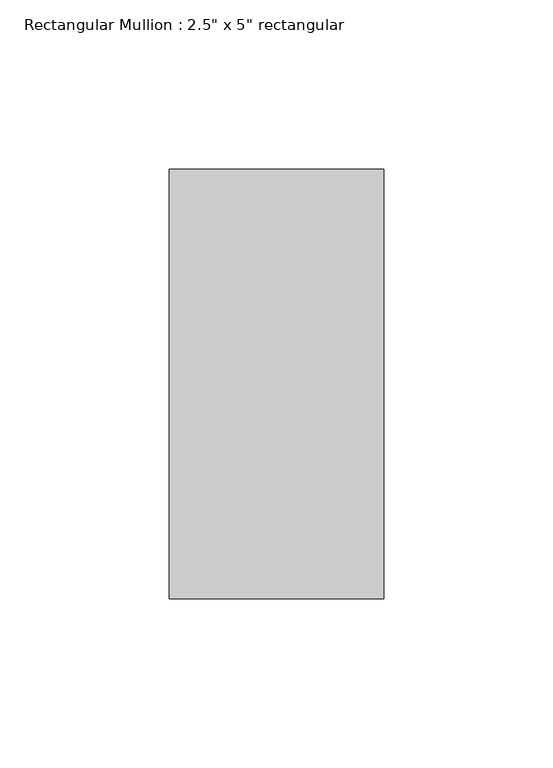
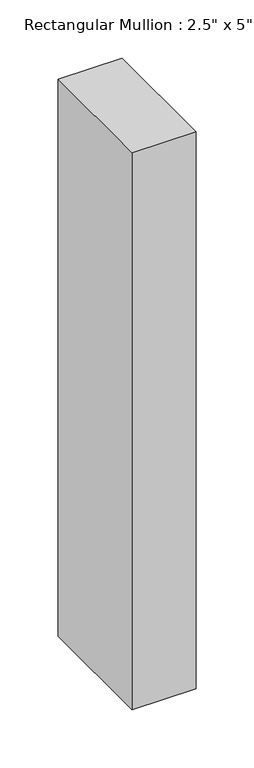
"""IFC4 building model written with IfcOpenShell, lengths in millimetres: member geometry."""

from ifc_helpers import new_model, si_unit, frame, origin, place, context, project, spatial, polyline, outline, extrude, source, transform, mapped, element, save


def member_6133cf7c(model_context):
    return source(origin(), model_context, "Body", "SweptSolid", [
        extrude(outline(polyline([(31.75, 63.5), (31.75, -63.5), (-31.75, -63.5), (-31.75, 63.5), (31.75, 63.5)])), frame((0.0, 0.0, -584.2173759), z_axis=(0.0, 0.0, 1.0), x_axis=(1.0, 0.0, 0.0)), (0.0, 0.0, 1.0), 584.2173759),
    ])


if __name__ == "__main__":
    model = new_model("IFC4")
    model_context = context("Model", 3, world=origin())
    ifc_project = project(units=[si_unit("LENGTHUNIT", "METRE", prefix="MILLI")], contexts=[model_context])
    site = spatial("IfcSite", under=ifc_project)
    building = spatial("IfcBuilding", under=site)
    placement = place(None, origin())
    member_shape = member_6133cf7c(model_context)
    element("IfcMember", 1, ObjectType="Rectangular Mullion : 2.5\" x 5\" rectangular", at=placement, inside=building, context=model_context, shape_type="MappedRepresentation", body=[
        mapped(member_shape, transform((0.0, 0.0, 0.0), x_axis=(1.0, 0.0, 0.0), y_axis=(0.0, 1.0, 0.0), z_axis=(0.0, 0.0, 1.0))),
    ])
    save(model, "model.ifc")

# Revit data of these elements
# Type "Rectangular Mullion : 2.5\" x 5\" rectangular"
#   built-in parameter 1007304 = 0.416667 (stored number, unit not read)
#   built-in parameter 1007301 = 0.104167 (stored number, unit not read)
#   built-in parameter 1007300 = 0.104167 (stored number, unit not read)
# Element 1 (IfcMember, "Rectangular Mullion : 2.5\" x 5\" rectangular")
#   Materials on its faces: "Aluminum"
# Materials
#   "Aluminum": class "Metal", colour RGB 247 247 247, transparency 0, Description = "Aluminum 6061", Cost = 0
